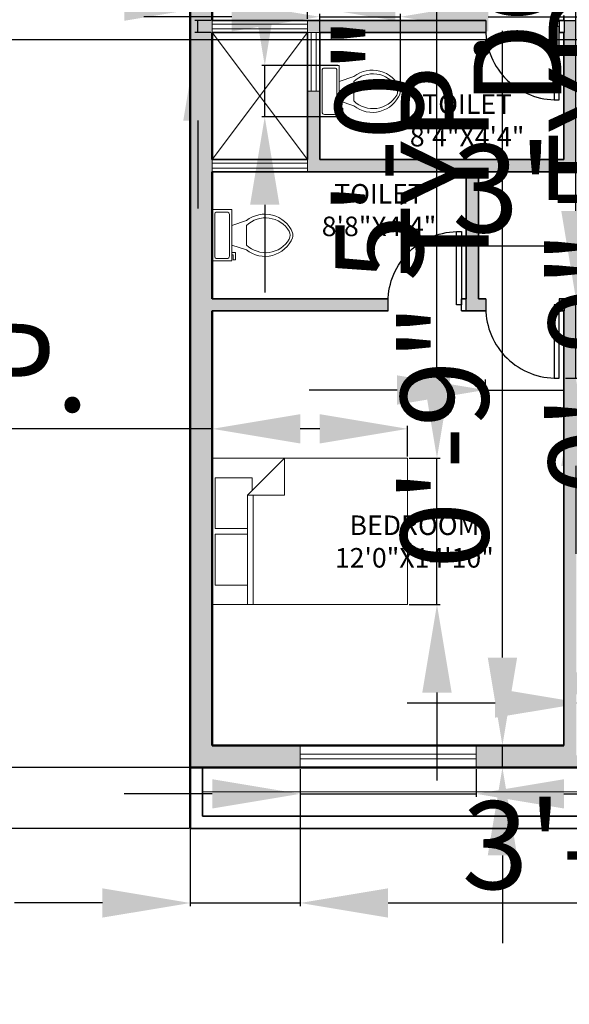
# Model space of a CAD drawing. Units: inches. Extents: x -299 to 1164, y -2 to 940.
# Tile 2 of 11: x 189 to 414, y 86 to 490. Entities that reach past the tile are written whole.
import ezdxf

# ---------------------------------------------------------------- set-up
doc = ezdxf.new("R2010")
doc.units = ezdxf.units.IN
for name, color, linetype, lineweight in [('A-AREA-IDEN', 3, 'Continuous', 25), ('A-FLOR-FIXT', 8, 'Continuous', 18), ('A-FLOR-OPEN', 7, 'Continuous', 13), ('A-FURN', 8, 'Continuous', 18), ('C-SITE-PVMT', 7, 'Continuous', 18), ('C-SITE-WALL', 7, 'Continuous', 35), ('dimensions', 191, 'Continuous', 18), ('doors', 20, 'Continuous', 25), ('inner walls', 7, 'Continuous', 35), ('outer walls', 7, 'Continuous', 50), ('windows', 130, 'Continuous', 18)]:
    doc.layers.add(name, color=color, linetype=linetype, lineweight=lineweight)
doc.layers.add('A-WALL-PATT', color=240, linetype='Continuous', lineweight=13, true_color=0xed1f24)
doc.styles.get("Standard").update_dxf_attribs({"font": 'arial.ttf'})
doc.dimstyles.new('ISO-25', dxfattribs={"dimtxt": 36, "dimasz": 36, "dimexe": 1.25, "dimexo": 0.625, "dimtad": 1, "dimlunit": 3, "dimtxsty": 'Standard', "dimcen": 2.5, "dimazin": 0, "dimtfac": 1, "dimtmove": 0, "dimatfit": 3, "dimfxl": 1, "dimarcsym": 0})

# ---------------------------------------------------------------- blocks, each defined once
blk = doc.blocks.new('Bed - Queen')
for p, q in [((0, -80.00003), (0, 0)), ((0, 0), (59.99999, 0)), ((59.99999, 0), (59.99999, -80.00003)), ((7.99999, -1.2), (28.79998, -1.2)), ((7.99999, -14.4), (7.99999, -1.2)), ((28.79998, -1.2), (28.79998, -14.4)), ((31.19999, -1.2), (51.99999, -1.2)), ((31.19999, -14.4), (31.19999, -1.2)), ((51.99999, -1.2), (51.99999, -16.4)), ((0, -14.4), (44.8, -14.4)), ((59.99999, -29.6), (44.8, -14.4)), ((44.8, -14.4), (44.8, -29.6)), ((44.8, -16.8), (0, -16.8)), ((51.99999, -16.4), (46.79936, -16.4)), ((44.8, -29.6), (59.99999, -29.6)), ((59.99999, -80.00003), (0, -80.00003))]:
    blk.add_line(p, q)
blk = doc.blocks.new('*U12')
for p, q in [((9.5, -6), (9.5, -2)), ((-8, -8.5), (-8, -8)), ((-7, -8), (-7, -9.5)), ((-4, -8), (-6, -14)), ((4, -8), (6, -14)), ((-10, -8.5), (-8, -8.5)), ((-10, -9.5), (-10, -8.5)), ((-7, -9.5), (-10, -9.5)), ((4, -14), (-4, -14))]:
    blk.add_line(p, q)
blk.add_lwpolyline([(10.5, -8), (10.5, 0), (-10.5, 0), (-10.5, -8)], close=True)
for points in [[(-9.5, -2), (-9.5, -6)], [(8.5, -1), (-8.5, -1)], [(-8.5, -7), (8.5, -7)]]:
    blk.add_lwpolyline(points)
for centre, radius, start, end in [((-8.62, -1.88), 0.884, 81.8699, 188.1301), ((8.62, -1.88), 0.884, 351.8699, 98.1301), ((-8.62, -6.12), 0.884, 171.8699, 278.1301), ((8.62, -6.12), 0.884, 261.8699, 8.1301), ((3.52, -21.58), 12.17, 141.4691, 247.9714), ((4.2, -21.82), 11.33, 136.3677, 238.9468), ((-3.52, -21.58), 12.17, 292.0284, 38.5307), ((-4.2, -21.82), 11.33, 301.053, 43.6321), ((0, -27.88), 4, 245.7318, 294.2682), ((0, -29), 4, 254.8605, 285.1395)]:
    blk.add_arc(centre, radius, start, end)
blk = doc.blocks.new('DOOR-30IN')
for p, q in [((0.03, 32.5), (0.03, 27.5)), ((30.03, 32.5), (30.03, 27.5)), ((32.03, 32.5), (32.03, 27.5))]:
    blk.add_line(p, q)
blk.add_lwpolyline([(28.03, 0), (30.03, 0), (30.03, 30), (28.03, 30)], close=True)
blk.add_arc((28.76, 28.75), 28.76, 177.5089, 268.5412)
blk = doc.blocks.new('WIN-39IN-VENT')
for p, q in [((0, 5), (0, 0)), ((39, 5), (0, 5)), ((39, 0), (39, 5)), ((0, 3.5), (39, 3.5)), ((0, 1.5), (39, 1.5)), ((0, 0), (39, 0))]:
    blk.add_line(p, q)
blk = doc.blocks.new('WIN-72IN')
for p, q in [((0, 5.5), (72, 5.5)), ((0, 3.5), (72, 3.5))]:
    blk.add_line(p, q)
blk.add_lwpolyline([(0, 0), (72, 0), (72, 9), (0, 9)], close=True)
blk = doc.blocks.new('*D25')
at = {"layer": 'Defpoints', "color": 0, "transparency": 16777216}
for p in [(443.65, 597.1), (453.38, 597.1), (443.65, 532.21)]:
    blk.add_point(p, dxfattribs=at)
at = {"layer": 'dimensions', "color": 0, "lineweight": -2, "transparency": 16777216}
for p, q in [((453.38, 633.1), (453.38, 916.77)), ((444.27, 597.1), (454.63, 597.1)), ((453.38, 532.21), (453.38, 597.1)), ((444.27, 532.21), (454.63, 532.21)), ((453.38, 496.21), (453.38, 460.21))]:
    blk.add_line(p, q, dxfattribs=at)
at = {"layer": 'dimensions', "color": 0, "transparency": 16777216}
for points in [[(447.38, 633.1), (459.38, 633.1), (453.38, 597.1)], [(447.38, 496.21), (459.38, 496.21), (453.38, 532.21)]]:
    blk.add_solid(points, dxfattribs=at)
at = {"layer": 'dimensions', "color": 0, "transparency": 16777216, "insert": (434.13, 792.94), "char_height": 36, "attachment_point": 5, "rotation": 90}
blk.add_mtext('SOFA 5\'-5"', dxfattribs=at)
blk = doc.blocks.new('*D27')
at = {"layer": 'Defpoints', "color": 0, "transparency": 16777216}
for p in [(412.07, 375.49), (416.95, 375.49), (412.07, 342.99)]:
    blk.add_point(p, dxfattribs=at)
at = {"layer": 'dimensions', "color": 0, "lineweight": -2, "transparency": 16777216}
for p, q in [((416.95, 411.49), (416.95, 915.12)), ((412.7, 375.49), (418.2, 375.49)), ((416.95, 342.99), (416.95, 375.49)), ((412.7, 342.99), (418.2, 342.99)), ((416.95, 306.99), (416.95, 270.99))]:
    blk.add_line(p, q, dxfattribs=at)
at = {"layer": 'dimensions', "color": 0, "transparency": 16777216}
for points in [[(410.95, 411.49), (422.95, 411.49), (416.95, 375.49)], [(410.95, 306.99), (422.95, 306.99), (416.95, 342.99)]]:
    blk.add_solid(points, dxfattribs=at)
at = {"layer": 'dimensions', "color": 0, "transparency": 16777216, "insert": (397.69, 681.3), "char_height": 36, "attachment_point": 5, "rotation": 90}
blk.add_mtext('DOOR 2\'-8 1/2" TYP.', dxfattribs=at)
blk = doc.blocks.new('*D28')
at = {"layer": 'Defpoints', "color": 0, "transparency": 16777216}
for p in [(379.74, 342.99), (412.07, 342.99), (412.07, 338.11)]:
    blk.add_point(p, dxfattribs=at)
at = {"layer": 'dimensions', "color": 0, "lineweight": -2, "transparency": 16777216}
for p, q in [((379.74, 342.36), (379.74, 336.86)), ((412.07, 342.36), (412.07, 336.86)), ((343.74, 338.11), (307.74, 338.11)), ((379.74, 338.11), (412.07, 338.11)), ((448.07, 338.11), (789.26, 338.11))]:
    blk.add_line(p, q, dxfattribs=at)
at = {"layer": 'dimensions', "color": 0, "transparency": 16777216}
for points in [[(343.74, 344.11), (343.74, 332.11), (379.74, 338.11)], [(448.07, 344.11), (448.07, 332.11), (412.07, 338.11)]]:
    blk.add_solid(points, dxfattribs=at)
at = {"layer": 'dimensions', "color": 0, "transparency": 16777216, "insert": (636.66, 357.35), "char_height": 36, "attachment_point": 5}
blk.add_mtext('2\'-8 1/2" TYP.', dxfattribs=at)
blk = doc.blocks.new('*D29')
at = {"layer": 'Defpoints', "color": 0, "transparency": 16777216}
for p in [(304.07, 183.49), (376.07, 183.49), (376.07, 172.69)]:
    blk.add_point(p, dxfattribs=at)
at = {"layer": 'dimensions', "color": 0, "lineweight": -2, "transparency": 16777216}
for p, q in [((304.07, 182.86), (304.07, 171.44)), ((376.07, 182.86), (376.07, 171.44)), ((268.07, 172.69), (232.07, 172.69)), ((304.07, 172.69), (376.07, 172.69)), ((412.07, 172.69), (904.87, 172.69))]:
    blk.add_line(p, q, dxfattribs=at)
at = {"layer": 'dimensions', "color": 0, "transparency": 16777216}
for points in [[(268.07, 178.69), (268.07, 166.69), (304.07, 172.69)], [(412.07, 178.69), (412.07, 166.69), (376.07, 172.69)]]:
    blk.add_solid(points, dxfattribs=at)
at = {"layer": 'dimensions', "color": 0, "transparency": 16777216, "insert": (676.47, 191.94), "char_height": 36, "attachment_point": 5}
blk.add_mtext('WINDOW 6\'-0" TYP.', dxfattribs=at)
blk = doc.blocks.new('*D30')
at = {"layer": 'Defpoints', "color": 0, "transparency": 16777216}
for p in [(376.07, 192.49), (386.87, 192.49), (376.07, 183.49)]:
    blk.add_point(p, dxfattribs=at)
at = {"layer": 'dimensions', "color": 0, "lineweight": -2, "transparency": 16777216}
for p, q in [((386.87, 228.49), (386.87, 485.18)), ((376.7, 192.49), (388.12, 192.49)), ((386.87, 183.49), (386.87, 192.49)), ((376.7, 183.49), (388.12, 183.49)), ((386.87, 147.49), (386.87, 111.49))]:
    blk.add_line(p, q, dxfattribs=at)
at = {"layer": 'dimensions', "color": 0, "transparency": 16777216}
for points in [[(380.87, 228.49), (392.87, 228.49), (386.87, 192.49)], [(380.87, 147.49), (392.87, 147.49), (386.87, 183.49)]]:
    blk.add_solid(points, dxfattribs=at)
at = {"layer": 'dimensions', "color": 0, "transparency": 16777216, "insert": (367.87, 374.83), "char_height": 36, "attachment_point": 5, "rotation": 90}
blk.add_mtext('0\'-9" TYP.', dxfattribs=at)
blk = doc.blocks.new('*D31')
at = {"layer": 'Defpoints', "color": 0, "transparency": 16777216}
for p in [(268.07, 322.2), (268.07, 310.2), (348.07, 310.2)]:
    blk.add_point(p, dxfattribs=at)
at = {"layer": 'dimensions', "color": 0, "lineweight": -2, "transparency": 16777216}
for p, q in [((268.07, 310.83), (268.07, 323.45)), ((348.07, 310.83), (348.07, 323.45)), ((268.07, 322.2), (-298.74, 322.2)), ((312.07, 322.2), (304.07, 322.2))]:
    blk.add_line(p, q, dxfattribs=at)
at = {"layer": 'dimensions', "color": 0, "transparency": 16777216}
for points in [[(304.07, 328.2), (304.07, 316.2), (268.07, 322.2)], [(312.07, 328.2), (312.07, 316.2), (348.07, 322.2)]]:
    blk.add_solid(points, dxfattribs=at)
at = {"layer": 'dimensions', "color": 0, "transparency": 16777216, "insert": (-33.34, 342.55), "char_height": 36, "attachment_point": 5}
blk.add_mtext('QUEEN BED 6\'-8" TYP.', dxfattribs=at)
blk = doc.blocks.new('*D32')
at = {"layer": 'Defpoints', "color": 0, "transparency": 16777216}
for p in [(348.07, 310.2), (360.07, 310.2), (348.07, 250.2)]:
    blk.add_point(p, dxfattribs=at)
at = {"layer": 'dimensions', "color": 0, "lineweight": -2, "transparency": 16777216}
for p, q in [((360.07, 346.2), (360.07, 602.89)), ((348.7, 310.2), (361.32, 310.2)), ((360.07, 250.2), (360.07, 310.2)), ((348.7, 250.2), (361.32, 250.2)), ((360.07, 214.2), (360.07, 178.2))]:
    blk.add_line(p, q, dxfattribs=at)
at = {"layer": 'dimensions', "color": 0, "transparency": 16777216}
for points in [[(354.07, 346.2), (366.07, 346.2), (360.07, 310.2)], [(354.07, 214.2), (366.07, 214.2), (360.07, 250.2)]]:
    blk.add_solid(points, dxfattribs=at)
at = {"layer": 'dimensions', "color": 0, "transparency": 16777216, "insert": (341.07, 492.55), "char_height": 36, "attachment_point": 5, "rotation": 90}
blk.add_mtext('5\'-0" TYP.', dxfattribs=at)
blk = doc.blocks.new('*D33')
at = {"layer": 'Defpoints', "color": 0, "transparency": 16777216}
for p in [(419.84, 213.49), (443.84, 213.49), (443.84, 209.89)]:
    blk.add_point(p, dxfattribs=at)
at = {"layer": 'dimensions', "color": 0, "lineweight": -2, "transparency": 16777216}
for p, q in [((383.84, 209.89), (347.84, 209.89)), ((419.84, 212.86), (419.84, 208.64)), ((419.84, 209.89), (443.84, 209.89)), ((443.84, 212.86), (443.84, 208.64)), ((479.84, 209.89), (970.68, 209.89))]:
    blk.add_line(p, q, dxfattribs=at)
at = {"layer": 'dimensions', "color": 0, "transparency": 16777216}
for points in [[(383.84, 215.89), (383.84, 203.89), (419.84, 209.89)], [(479.84, 215.89), (479.84, 203.89), (443.84, 209.89)]]:
    blk.add_solid(points, dxfattribs=at)
at = {"layer": 'dimensions', "color": 0, "transparency": 16777216, "insert": (743.26, 229.13), "char_height": 36, "attachment_point": 5}
blk.add_mtext('GLAZING 2\'-0" TYP.', dxfattribs=at)
blk = doc.blocks.new('*D34')
at = {"layer": 'Defpoints', "color": 0, "transparency": 16777216}
for p in [(443.84, 222.49), (447.44, 222.49), (443.84, 213.49)]:
    blk.add_point(p, dxfattribs=at)
at = {"layer": 'dimensions', "color": 0, "lineweight": -2, "transparency": 16777216}
for p, q in [((447.44, 258.49), (447.44, 515.18)), ((444.47, 222.49), (448.69, 222.49)), ((447.44, 213.49), (447.44, 222.49)), ((444.47, 213.49), (448.69, 213.49)), ((447.44, 177.49), (447.44, 141.49))]:
    blk.add_line(p, q, dxfattribs=at)
at = {"layer": 'dimensions', "color": 0, "transparency": 16777216}
for points in [[(441.44, 258.49), (453.44, 258.49), (447.44, 222.49)], [(441.44, 177.49), (453.44, 177.49), (447.44, 213.49)]]:
    blk.add_solid(points, dxfattribs=at)
at = {"layer": 'dimensions', "color": 0, "transparency": 16777216, "insert": (428.44, 404.83), "char_height": 36, "attachment_point": 5, "rotation": 90}
blk.add_mtext('0\'-9" TYP.', dxfattribs=at)
blk = doc.blocks.new('*D35')
at = {"layer": 'Defpoints', "color": 0, "transparency": 16777216}
for p in [(307.07, 495.34), (268.07, 489.49), (307.07, 489.49)]:
    blk.add_point(p, dxfattribs=at)
at = {"layer": 'dimensions', "color": 0, "lineweight": -2, "transparency": 16777216}
for p, q in [((268.07, 490.11), (268.07, 496.59)), ((307.07, 490.11), (307.07, 496.59)), ((232.07, 495.34), (196.07, 495.34)), ((268.07, 495.34), (307.07, 495.34)), ((343.07, 495.34), (749.73, 495.34))]:
    blk.add_line(p, q, dxfattribs=at)
at = {"layer": 'dimensions', "color": 0, "transparency": 16777216}
for points in [[(232.07, 501.34), (232.07, 489.34), (268.07, 495.34)], [(343.07, 501.34), (343.07, 489.34), (307.07, 495.34)]]:
    blk.add_solid(points, dxfattribs=at)
at = {"layer": 'dimensions', "color": 0, "transparency": 16777216, "insert": (564.4, 514.36), "char_height": 36, "attachment_point": 5}
blk.add_mtext('VENT 3\'-3" TYP.', dxfattribs=at)
blk = doc.blocks.new('*D36')
at = {"layer": 'Defpoints', "color": 0, "transparency": 16777216}
for p in [(262.22, 489.49), (268.07, 489.49), (268.07, 484.49)]:
    blk.add_point(p, dxfattribs=at)
at = {"layer": 'dimensions', "color": 0, "lineweight": -2, "transparency": 16777216}
for p, q in [((262.22, 525.49), (262.22, 782.18)), ((267.45, 489.49), (260.97, 489.49)), ((262.22, 484.49), (262.22, 489.49)), ((267.45, 484.49), (260.97, 484.49)), ((262.22, 448.49), (262.22, 412.49))]:
    blk.add_line(p, q, dxfattribs=at)
at = {"layer": 'dimensions', "color": 0, "transparency": 16777216}
for points in [[(256.22, 525.49), (268.22, 525.49), (262.22, 489.49)], [(256.22, 448.49), (268.22, 448.49), (262.22, 484.49)]]:
    blk.add_solid(points, dxfattribs=at)
at = {"layer": 'dimensions', "color": 0, "transparency": 16777216, "insert": (243.22, 671.83), "char_height": 36, "attachment_point": 5, "rotation": 90}
blk.add_mtext('0\'-5" TYP.', dxfattribs=at)
blk = doc.blocks.new('*D47')
at = {"layer": 'Defpoints', "color": 0, "transparency": 16777216}
for p in [(502.07, 668.99), (466.07, 222.49), (502.07, 222.49)]:
    blk.add_point(p, dxfattribs=at)
at = {"layer": 'dimensions', "color": 0, "lineweight": -2, "transparency": 16777216}
for p, q in [((466.07, 223.11), (466.07, 670.24)), ((502.07, 223.11), (502.07, 670.24)), ((430.07, 668.99), (394.07, 668.99)), ((466.07, 668.99), (502.07, 668.99)), ((538.07, 668.99), (670.99, 668.99))]:
    blk.add_line(p, q, dxfattribs=at)
at = {"layer": 'dimensions', "color": 0, "transparency": 16777216}
for points in [[(430.07, 674.99), (430.07, 662.99), (466.07, 668.99)], [(538.07, 674.99), (538.07, 662.99), (502.07, 668.99)]]:
    blk.add_solid(points, dxfattribs=at)
at = {"layer": 'dimensions', "color": 0, "transparency": 16777216, "insert": (622.53, 688.01), "char_height": 36, "attachment_point": 5}
blk.add_mtext('3\'-0"', dxfattribs=at)
blk = doc.blocks.new('*D49')
at = {"layer": 'Defpoints', "color": 0, "transparency": 16777216}
for p in [(259.07, 183.49), (304.07, 183.49), (304.07, 127.99)]:
    blk.add_point(p, dxfattribs=at)
at = {"layer": 'dimensions', "color": 0, "lineweight": -2, "transparency": 16777216}
for p, q in [((259.07, 182.86), (259.07, 126.74)), ((304.07, 182.86), (304.07, 126.74)), ((223.07, 127.99), (187.07, 127.99)), ((259.07, 127.99), (304.07, 127.99)), ((340.07, 127.99), (472.99, 127.99))]:
    blk.add_line(p, q, dxfattribs=at)
at = {"layer": 'dimensions', "color": 0, "transparency": 16777216}
for points in [[(223.07, 133.99), (223.07, 121.99), (259.07, 127.99)], [(340.07, 133.99), (340.07, 121.99), (304.07, 127.99)]]:
    blk.add_solid(points, dxfattribs=at)
at = {"layer": 'dimensions', "color": 0, "transparency": 16777216, "insert": (424.53, 147.01), "char_height": 36, "attachment_point": 5}
blk.add_mtext('3\'-9"', dxfattribs=at)
blk = doc.blocks.new('*D50')
at = {"layer": 'Defpoints', "color": 0, "transparency": 16777216}
for p in [(177.57, 183.49), (259.07, 183.49), (259.07, 158.49)]:
    blk.add_point(p, dxfattribs=at)
at = {"layer": 'dimensions', "color": 0, "lineweight": -2, "transparency": 16777216}
for p, q in [((177.57, 219.49), (177.57, 353.05)), ((258.45, 183.49), (176.32, 183.49)), ((177.57, 158.49), (177.57, 183.49)), ((258.45, 158.49), (176.32, 158.49)), ((177.57, 122.49), (177.57, 86.49))]:
    blk.add_line(p, q, dxfattribs=at)
at = {"layer": 'dimensions', "color": 0, "transparency": 16777216}
for points in [[(171.57, 219.49), (183.57, 219.49), (177.57, 183.49)], [(171.57, 122.49), (183.57, 122.49), (177.57, 158.49)]]:
    blk.add_solid(points, dxfattribs=at)
at = {"layer": 'dimensions', "color": 0, "transparency": 16777216, "insert": (158.87, 304.27), "char_height": 36, "attachment_point": 5, "rotation": 90}
blk.add_mtext('2\'-1"', dxfattribs=at)
blk = doc.blocks.new('*D53')
at = {"layer": 'Defpoints', "color": 0, "transparency": 16777216}
for p in [(177.57, 553.49), (586.07, 553.49), (586.07, 481.49)]:
    blk.add_point(p, dxfattribs=at)
at = {"layer": 'dimensions', "color": 0, "lineweight": -2, "transparency": 16777216}
for p, q in [((177.57, 589.49), (177.57, 722.63)), ((585.45, 553.49), (176.32, 553.49)), ((177.57, 481.49), (177.57, 553.49)), ((585.45, 481.49), (176.32, 481.49)), ((177.57, 445.49), (177.57, 409.49))]:
    blk.add_line(p, q, dxfattribs=at)
at = {"layer": 'dimensions', "color": 0, "transparency": 16777216}
for points in [[(171.57, 589.49), (183.57, 589.49), (177.57, 553.49)], [(171.57, 445.49), (183.57, 445.49), (177.57, 481.49)]]:
    blk.add_solid(points, dxfattribs=at)
at = {"layer": 'dimensions', "color": 0, "transparency": 16777216, "insert": (158.57, 674.06), "char_height": 36, "attachment_point": 5, "rotation": 90}
blk.add_mtext('6\'-0"', dxfattribs=at)
blk = doc.blocks.new('*D54')
at = {"layer": 'Defpoints', "color": 0, "transparency": 16777216}
for p in [(345.07, 490.99), (312.07, 460.49), (345.07, 460.49)]:
    blk.add_point(p, dxfattribs=at)
at = {"layer": 'dimensions', "color": 0, "lineweight": -2, "transparency": 16777216}
for p, q in [((312.07, 461.11), (312.07, 492.24)), ((345.07, 461.11), (345.07, 492.24)), ((276.07, 490.99), (240.07, 490.99)), ((312.07, 490.99), (345.07, 490.99)), ((381.07, 490.99), (514.63, 490.99))]:
    blk.add_line(p, q, dxfattribs=at)
at = {"layer": 'dimensions', "color": 0, "transparency": 16777216}
for points in [[(276.07, 496.99), (276.07, 484.99), (312.07, 490.99)], [(381.07, 496.99), (381.07, 484.99), (345.07, 490.99)]]:
    blk.add_solid(points, dxfattribs=at)
at = {"layer": 'dimensions', "color": 0, "transparency": 16777216, "insert": (465.85, 509.99), "char_height": 36, "attachment_point": 5}
blk.add_mtext('2\'-9"', dxfattribs=at)
blk = doc.blocks.new('*D55')
at = {"layer": 'Defpoints', "color": 0, "transparency": 16777216}
for p in [(289.57, 470.99), (320.07, 470.99), (320.07, 449.99)]:
    blk.add_point(p, dxfattribs=at)
at = {"layer": 'dimensions', "color": 0, "lineweight": -2, "transparency": 16777216}
for p, q in [((289.57, 506.99), (289.57, 636.55)), ((319.45, 470.99), (288.32, 470.99)), ((289.57, 449.99), (289.57, 470.99)), ((319.45, 449.99), (288.32, 449.99)), ((289.57, 413.99), (289.57, 377.99))]:
    blk.add_line(p, q, dxfattribs=at)
at = {"layer": 'dimensions', "color": 0, "transparency": 16777216}
for points in [[(283.57, 506.99), (295.57, 506.99), (289.57, 470.99)], [(283.57, 413.99), (295.57, 413.99), (289.57, 449.99)]]:
    blk.add_solid(points, dxfattribs=at)
at = {"layer": 'dimensions', "color": 0, "transparency": 16777216, "insert": (270.57, 589.77), "char_height": 36, "attachment_point": 5, "rotation": 90}
blk.add_mtext('1\'-9"', dxfattribs=at)
blk = doc.blocks.new('*D57')
at = {"layer": 'Defpoints', "color": 0, "transparency": 16777216}
for p in [(541.07, 427.49), (577.07, 427.49), (541.07, 396.99)]:
    blk.add_point(p, dxfattribs=at)
at = {"layer": 'dimensions', "color": 0, "lineweight": -2, "transparency": 16777216}
for p, q in [((541.07, 426.86), (541.07, 395.74)), ((577.07, 426.86), (577.07, 395.74)), ((505.07, 396.99), (372.15, 396.99)), ((577.07, 396.99), (541.07, 396.99)), ((613.07, 396.99), (649.07, 396.99))]:
    blk.add_line(p, q, dxfattribs=at)
at = {"layer": 'dimensions', "color": 0, "transparency": 16777216}
for points in [[(505.07, 402.99), (505.07, 390.99), (541.07, 396.99)], [(613.07, 402.99), (613.07, 390.99), (577.07, 396.99)]]:
    blk.add_solid(points, dxfattribs=at)
at = {"layer": 'dimensions', "color": 0, "transparency": 16777216, "insert": (420.61, 416.01), "char_height": 36, "attachment_point": 5}
blk.add_mtext('3\'-0"', dxfattribs=at)

msp = doc.modelspace()

# ---------------------------------------------------------------- hatches: boundary and pattern name
at = {"layer": 'A-WALL-PATT'}
h = msp.add_hatch(color=256, dxfattribs=at)
h.dxf.hatch_style = 1
h.paths.add_polyline_path([(312.071, 460.489), (307.071, 460.489), (307.071, 432.489), (307.071, 427.489), (372.071, 427.489), (372.071, 375.489), (372.071, 370.489), (380.071, 370.489, -0.0217424), (380.071, 372.989), (380.071, 375.489), (377.071, 375.489), (377.071, 427.489), (417.071, 427.489), (417.071, 489.489), (412.071, 489.489), (412.071, 484.489), (412.071, 432.489), (312.071, 432.489)], flags=17)
h.paths.add_polyline_path([(340.071, 372.989, -0.0217424), (340.071, 375.489), (268.071, 375.489), (268.071, 427.489), (268.071, 432.489), (268.071, 484.489), (268.071, 489.489), (268.071, 629.489), (412.071, 629.489), (412.071, 527.563, -0.0185322), (414.571, 527.489), (417.071, 527.489), (417.071, 629.489), (581.071, 629.489), (581.071, 553.489), (586.071, 553.489), (586.071, 629.489), (730.071, 629.489), (730.071, 405.489), (713.071, 405.489), (713.071, 396.489), (739.071, 396.489), (739.071, 638.489), (259.071, 638.489), (259.071, 183.489), (304.071, 183.489), (304.071, 192.489), (268.071, 192.489), (268.071, 370.489), (340.071, 370.489)])
h.paths.add_polyline_path([(417.071, 188.489), (417.071, 213.489), (461.071, 213.489), (461.071, 188.489)], flags=16)
h.paths.add_polyline_path([(586.071, 313.578), (577.071, 313.578), (577.071, 311.489), (575.54, 311.489), (575.54, 302.489), (586.071, 302.489)], flags=16)
h.paths.add_polyline_path([(586.071, 405.489), (586.071, 481.489), (581.071, 481.489), (581.071, 432.489), (499.071, 432.489), (499.071, 427.489), (577.071, 427.489), (577.071, 385.578), (586.071, 385.578), (586.071, 396.489)], flags=17)
h.paths.add_polyline_path([(641.071, 405.489), (624.071, 405.489, -0.0333689), (624.071, 400.989), (624.071, 396.489), (641.071, 396.489)], flags=17)
h.paths.add_polyline_path([(491.866, 222.489), (491.866, 213.489), (586.071, 213.489), (586.071, 222.489)])
edge = h.paths.add_edge_path()
edge.add_line((467.866, 213.489), (467.866, 222.489))
edge.add_line((467.866, 222.489), (466.071, 222.489))
edge.add_line((466.071, 222.489), (466.071, 302.489))
edge.add_line((466.071, 302.489), (527.54, 302.489))
edge.add_line((527.54, 302.489), (527.54, 311.489))
edge.add_line((527.54, 311.489), (449.071, 311.489))
edge.add_line((449.071, 311.489), (449.071, 308.989))
edge.add_arc((420.339, 307.739), 28.759, -2.4911, 2.4911, ccw=False)
edge.add_line((449.071, 306.489), (461.071, 306.489))
edge.add_line((461.071, 306.489), (461.071, 222.489))
edge.add_line((461.071, 222.489), (443.844, 222.489))
edge.add_line((443.844, 222.489), (443.844, 213.489))
edge.add_line((443.844, 213.489), (419.844, 213.489))
edge.add_line((419.844, 213.489), (419.844, 222.489))
edge.add_line((419.844, 222.489), (417.071, 222.489))
edge.add_line((417.071, 222.489), (417.071, 306.489))
edge.add_line((417.071, 306.489), (417.071, 311.489))
edge.add_line((417.071, 311.489), (417.071, 375.489))
edge.add_line((417.071, 375.489), (412.071, 375.489))
edge.add_line((412.071, 375.489), (412.071, 370.489))
edge.add_line((412.071, 370.489), (412.071, 192.489))
edge.add_line((412.071, 192.489), (376.071, 192.489))
edge.add_line((376.071, 192.489), (376.071, 183.489))
edge.add_line((376.071, 183.489), (412.071, 183.489))
edge.add_line((412.071, 183.489), (466.071, 183.489))
edge.add_line((466.071, 183.489), (466.071, 213.489))
edge.add_line((466.071, 213.489), (467.866, 213.489))
h = msp.add_hatch(color=256, dxfattribs=at)
h.dxf.hatch_style = 1
h.paths.add_polyline_path([(380.071, 489.489), (307.071, 489.489), (307.071, 484.489), (312.071, 484.489), (380.071, 484.489, -0.0217424), (380.071, 486.989)])

# ---------------------------------------------------------------- linework, layer by layer
at = {"layer": 'A-FLOR-OPEN'}
for p, q in [((268.071, 484.489), (307.071, 432.489)), ((268.071, 432.489), (307.071, 484.489))]:
    msp.add_line(p, q, dxfattribs=at)
at = {"layer": 'C-SITE-PVMT'}
msp.add_line((264.071, 173.489), (466.071, 173.489), dxfattribs=at)
at = {"layer": 'C-SITE-WALL'}
for p, q in [((264.071, 183.489), (264.071, 163.489)), ((264.071, 163.489), (654.071, 163.489)), ((259.071, 158.489), (654.071, 158.489))]:
    msp.add_line(p, q, dxfattribs=at)
at = {"layer": 'doors'}
msp.add_line((412.071, 489.489), (417.071, 489.489), dxfattribs=at)
at = {"layer": 'inner walls'}
for p, q in [((380.071, 489.489), (268.071, 489.489)), ((412.071, 489.489), (410.071, 489.489)), ((412.071, 491.489), (412.071, 489.489)), ((307.071, 484.489), (268.071, 484.489)), ((307.071, 484.489), (307.071, 432.489)), ((312.071, 484.489), (312.071, 432.489)), ((380.071, 484.489), (312.071, 484.489)), ((412.071, 484.489), (410.071, 484.489)), ((412.071, 484.489), (412.071, 432.489)), ((307.071, 432.489), (268.071, 432.489)), ((307.071, 432.489), (268.071, 432.489)), ((412.071, 432.489), (312.071, 432.489)), ((380.071, 432.489), (312.071, 432.489)), ((372.071, 427.489), (268.071, 427.489)), ((307.071, 427.489), (268.071, 427.489)), ((372.071, 427.489), (372.071, 375.489)), ((377.071, 427.489), (377.071, 375.489)), ((417.071, 427.489), (377.071, 427.489)), ((340.071, 375.489), (268.071, 375.489)), ((372.071, 375.489), (370.071, 375.489)), ((380.071, 375.489), (377.071, 375.489)), ((417.071, 375.489), (410.071, 375.489)), ((340.071, 370.489), (268.071, 370.489)), ((380.071, 370.489), (370.071, 370.489)), ((412.071, 370.489), (410.071, 370.489)), ((412.071, 370.489), (412.071, 192.489))]:
    msp.add_line(p, q, dxfattribs=at)
at = {"layer": 'outer walls'}
for p, q in [((259.071, 638.489), (259.071, 158.489)), ((268.071, 629.489), (268.071, 489.489)), ((268.071, 484.489), (268.071, 432.489)), ((268.071, 427.489), (268.071, 375.489)), ((268.071, 370.489), (268.071, 192.489)), ((412.071, 192.489), (268.071, 192.489)), ((412.071, 183.489), (259.071, 183.489)), ((466.071, 183.489), (412.071, 183.489))]:
    msp.add_line(p, q, dxfattribs=at)
at = {"layer": 'windows'}
for p, q in [((312.071, 484.489), (307.071, 484.489)), ((307.071, 484.489), (307.071, 460.489)), ((308.571, 484.489), (308.571, 460.489)), ((310.571, 484.489), (310.571, 460.489)), ((312.071, 460.489), (312.071, 484.489)), ((307.071, 460.489), (312.071, 460.489))]:
    msp.add_line(p, q, dxfattribs=at)

# ---------------------------------------------------------------- block references
at = {"layer": 'A-FLOR-FIXT', "rotation": 90}
for p in [(312.071, 460.489), (268.071, 401.489)]:
    msp.add_blockref('*U12', p, dxfattribs=at)
at = {"layer": 'A-FURN', "rotation": 90}
msp.add_blockref('Bed - Queen', (268.071, 250.202), dxfattribs=at)
at = {"layer": 'doors'}
for p in [(380.045, 456.989), (380.045, 342.989)]:
    msp.add_blockref('DOOR-30IN', p, dxfattribs=at)
at = {"layer": 'doors', "extrusion": (0, 0, -1), "zscale": -1, "rotation": 180}
msp.add_blockref('DOOR-30IN', (-340.045, 402.989), dxfattribs=at)
at = {"layer": 'windows'}
for name, p in [('WIN-39IN-VENT', (268.071, 484.489)), ('WIN-39IN-VENT', (268.071, 427.489)), ('WIN-72IN', (304.071, 183.489))]:
    msp.add_blockref(name, p, dxfattribs=at)

# ---------------------------------------------------------------- texts
at = {"layer": 'A-AREA-IDEN', "char_height": 8, "attachment_point": 1}
for s, insert in [('\\pxqc,t15;TOILET\\P8\'4"X4\'4"', (337.49, 459.216)), ('\\pxqc,t15;TOILET\\P8\'8"X4\'4"', (301.427, 422.469)), ('\\pxqc,t15;BEDROOM\\P12\'0"X14\'10"', (315.893, 286.71))]:
    msp.add_mtext_dynamic_manual_height_columns(s, width=69.83809, gutter_width=12.5, heights=[0], dxfattribs=dict(at, insert=insert))

# ---------------------------------------------------------------- dimensions: what is measured, and where the dimension line sits
at = {"layer": 'dimensions'}
for base, p1, p2, angle, text, picture, middle in [((453.378, 597.099), (443.646, 532.214), (443.646, 597.099), 90, 'SOFA <>', '*D25', (434.127, 792.936)), ((416.946, 375.489), (412.071, 342.989), (412.071, 375.489), 90, 'DOOR <> TYP.', '*D27', (397.695, 681.304)), ((262.221, 489.489), (268.071, 484.489), (268.071, 489.489), 90, '<> TYP.', '*D36', (243.215, 671.833)), ((360.071, 310.202), (348.071, 250.202), (348.071, 310.202), 90, '<> TYP.', '*D32', (341.065, 492.546)), ((447.444, 222.489), (443.844, 213.489), (443.844, 222.489), 90, '<> TYP.', '*D34', (428.438, 404.833)), ((386.871, 192.489), (376.071, 183.489), (376.071, 192.489), 90, '<> TYP.', '*D30', (367.865, 374.833)), ((268.071, 322.202), (348.071, 310.202), (268.071, 310.202), 180, 'QUEEN BED <> TYP.', '*D31', (-33.336, 342.546))]:
    dim = msp.add_linear_dim(base=base, p1=p1, p2=p2, angle=angle, text=text, dimstyle='ISO-25', override={"dimdec": 1, "dimlfac": 1, "dimrnd": 0, "dimzin": 1, "dimdsep": 46, "dimlunit": 4, "dimfrac": 2}, dxfattribs=at)
    dim.commit()
    dim.dimension.update_dxf_attribs({"geometry": picture, "text_midpoint": middle})
for base, p1, p2, angle, picture, middle in [((177.571, 553.489), (586.071, 481.489), (586.071, 553.489), 90, '*D53', (158.565, 674.061)), ((289.571, 470.989), (320.071, 449.989), (320.071, 470.989), 90, '*D55', (270.565, 589.768)), ((345.071, 490.989), (312.071, 460.489), (345.071, 460.489), 0.00004, '*D54', (465.852, 509.995)), ((541.071, 396.989), (577.071, 427.489), (541.071, 427.489), 180, '*D57', (420.61, 416.007)), ((177.571, 183.489), (259.071, 158.489), (259.071, 183.489), 90, '*D50', (158.872, 304.27))]:
    dim = msp.add_linear_dim(base=base, p1=p1, p2=p2, angle=angle, dimstyle='ISO-25', override={"dimdec": 1, "dimlfac": 1, "dimrnd": 0, "dimzin": 1, "dimdsep": 46, "dimlunit": 4, "dimfrac": 2}, dxfattribs=at)
    dim.commit()
    dim.dimension.update_dxf_attribs({"geometry": picture, "text_midpoint": middle})
for base, p1, p2, picture, middle in [((502.071, 668.989), (466.071, 222.489), (502.071, 222.489), '*D47', (622.532, 688.007)), ((304.071, 127.989), (259.071, 183.489), (304.071, 183.489), '*D49', (424.532, 147.007))]:
    dim = msp.add_linear_dim(base=base, p1=p1, p2=p2, dimstyle='ISO-25', override={"dimdec": 1, "dimlfac": 1, "dimrnd": 0, "dimzin": 1, "dimdsep": 46, "dimlunit": 4, "dimfrac": 2}, dxfattribs=at)
    dim.commit()
    dim.dimension.update_dxf_attribs({"geometry": picture, "text_midpoint": middle})
for base, p1, p2, text, picture, middle in [((307.071, 495.339), (268.071, 489.489), (307.071, 489.489), 'VENT <> TYP.', '*D35', (564.399, 514.357)), ((412.071, 338.114), (379.736, 342.989), (412.071, 342.989), '<> TYP.', '*D28', (636.665, 357.353)), ((443.844, 209.889), (419.844, 213.489), (443.844, 213.489), 'GLAZING <> TYP.', '*D33', (743.261, 229.128)), ((376.071, 172.689), (304.071, 183.489), (376.071, 183.489), 'WINDOW <> TYP.', '*D29', (676.471, 191.94))]:
    dim = msp.add_linear_dim(base=base, p1=p1, p2=p2, text=text, dimstyle='ISO-25', override={"dimdec": 1, "dimlfac": 1, "dimrnd": 0, "dimzin": 1, "dimdsep": 46, "dimlunit": 4, "dimfrac": 2}, dxfattribs=at)
    dim.commit()
    dim.dimension.update_dxf_attribs({"geometry": picture, "text_midpoint": middle})

doc.saveas('drawing.dxf')
